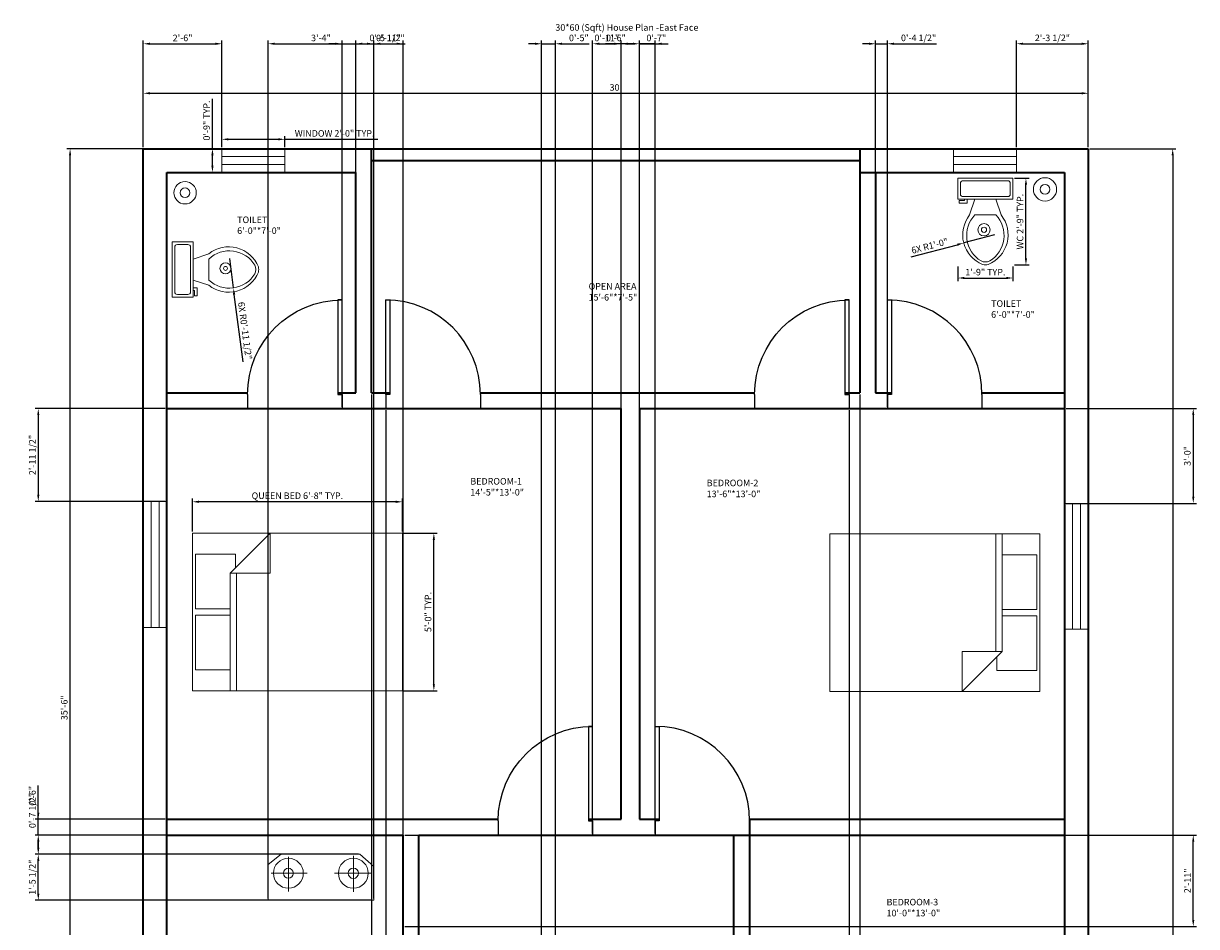
# Model space of a CAD drawing. Units: inches. Extents: x 2162 to 2610, y 1546 to 2356.
# Tile 3 of 3: x 2162 to 2609, y 2012 to 2356. Entities that reach past the tile are written whole.
import ezdxf

# ---------------------------------------------------------------- set-up
doc = ezdxf.new("R2010")
doc.units = ezdxf.units.IN
for name, color, linetype, lineweight in [('A-ANNO-DIMS', 2, 'Continuous', 18), ('A-ANNO-TEXT', 7, 'Continuous', 25), ('A-AREA-IDEN', 7, 'Continuous', 18), ('A-DOOR', 3, 'Continuous', 25), ('A-EQPM', 8, 'Continuous', 18), ('A-FLOR-FIXT', 9, 'Continuous', 18), ('A-FURN', 8, 'Continuous', 18), ('A-GLAZ', 4, 'Continuous', 18), ('A-WALL', 7, 'Continuous', 35)]:
    doc.layers.add(name, color=color, linetype=linetype, lineweight=lineweight)
doc.styles.get("Standard").update_dxf_attribs({"font": 'arial.ttf'})
doc.dimstyles.new('ISO-25', dxfattribs={"dimtxt": 2.5, "dimasz": 2.5, "dimexe": 1.25, "dimexo": 0.625, "dimtad": 1, "dimdec": 1, "dimlunit": 3, "dimtxsty": 'Standard', "dimcen": 2.5, "dimadec": 0, "dimazin": 0, "dimtfac": 1, "dimtdec": 1, "dimtmove": 0, "dimatfit": 3, "dimfxl": 1, "dimarcsym": 0})

# ---------------------------------------------------------------- blocks, each defined once
blk = doc.blocks.new('*U2')
for p, q in [((0, 0), (0, -6)), ((40, 0), (40, -6))]:
    blk.add_line(p, q)
blk.add_lwpolyline([(0, 0), (0, 40), (1.75, 40), (1.75, 0)], close=True)
blk.add_arc((0, 0), 40, 0, 90)
blk = doc.blocks.new('*D3')
at = {"layer": 'A-ANNO-DIMS', "color": 0, "lineweight": -2, "transparency": 16777216}
for p, q in [((2207.87, 2308.68), (2207.87, 2330.44)), ((2210.37, 2329.19), (2565.37, 2329.19)), ((2567.87, 2308.68), (2567.87, 2330.44))]:
    blk.add_line(p, q, dxfattribs=at)
at = {"layer": 'A-ANNO-DIMS', "color": 0, "transparency": 16777216}
for points in [[(2210.37, 2329.61), (2210.37, 2328.77), (2207.87, 2329.19)], [(2565.37, 2329.61), (2565.37, 2328.77), (2567.87, 2329.19)]]:
    blk.add_solid(points, dxfattribs=at)
at = {"layer": 'Defpoints', "color": 0, "transparency": 16777216}
for p in [(2567.87, 2329.19), (2207.87, 2308.05), (2567.87, 2308.05)]:
    blk.add_point(p, dxfattribs=at)
at = {"layer": 'A-ANNO-DIMS', "color": 0, "transparency": 16777216, "insert": (2387.87, 2331.09), "char_height": 2.5, "attachment_point": 5}
blk.add_mtext("30'", dxfattribs=at)
blk = doc.blocks.new('*D4')
at = {"layer": 'A-ANNO-DIMS', "color": 0, "lineweight": -2, "transparency": 16777216}
for p, q in [((2216.24, 2308.05), (2178.74, 2308.05)), ((2179.99, 1884.55), (2179.99, 2305.55)), ((2216.24, 1882.05), (2178.74, 1882.05))]:
    blk.add_line(p, q, dxfattribs=at)
at = {"layer": 'A-ANNO-DIMS', "color": 0, "transparency": 16777216}
for points in [[(2179.57, 2305.55), (2180.4, 2305.55), (2179.99, 2308.05)], [(2179.57, 1884.55), (2180.4, 1884.55), (2179.99, 1882.05)]]:
    blk.add_solid(points, dxfattribs=at)
at = {"layer": 'Defpoints', "color": 0, "transparency": 16777216}
for p in [(2179.99, 2308.05), (2216.87, 2308.05), (2216.87, 1882.05)]:
    blk.add_point(p, dxfattribs=at)
at = {"layer": 'A-ANNO-DIMS', "color": 0, "transparency": 16777216, "insert": (2178.09, 2095.05), "char_height": 2.5, "attachment_point": 5, "rotation": 90}
blk.add_mtext('35\'-6"', dxfattribs=at)
blk = doc.blocks.new('*D5')
at = {"layer": 'A-ANNO-DIMS', "color": 0, "lineweight": -2, "transparency": 16777216}
for p, q in [((2568.49, 2308.05), (2601.29, 2308.05)), ((2600.04, 2305.55), (2600.04, 1590.55)), ((2568.49, 1588.05), (2601.29, 1588.05))]:
    blk.add_line(p, q, dxfattribs=at)
at = {"layer": 'A-ANNO-DIMS', "color": 0, "transparency": 16777216}
for points in [[(2599.62, 2305.55), (2600.45, 2305.55), (2600.04, 2308.05)], [(2599.62, 1590.55), (2600.45, 1590.55), (2600.04, 1588.05)]]:
    blk.add_solid(points, dxfattribs=at)
at = {"layer": 'Defpoints', "color": 0, "transparency": 16777216}
for p in [(2567.87, 2308.05), (2567.87, 1588.05), (2600.04, 1588.05)]:
    blk.add_point(p, dxfattribs=at)
at = {"layer": 'A-ANNO-DIMS', "color": 0, "transparency": 16777216, "insert": (2598.14, 1948.05), "char_height": 2.5, "attachment_point": 5, "rotation": 90}
blk.add_mtext("60'", dxfattribs=at)
blk = doc.blocks.new('Bed - Queen')
for p, q in [((0, -80.00003), (0, 0)), ((0, 0), (59.99999, 0)), ((59.99999, 0), (59.99999, -80.00003)), ((7.99999, -1.2), (28.79998, -1.2)), ((7.99999, -14.4), (7.99999, -1.2)), ((28.79998, -1.2), (28.79998, -14.4)), ((31.19999, -1.2), (51.99999, -1.2)), ((31.19999, -14.4), (31.19999, -1.2)), ((51.99999, -1.2), (51.99999, -16.4)), ((0, -14.4), (44.8, -14.4)), ((44.8, -16.8), (0, -16.8)), ((59.99999, -29.6), (44.8, -14.4)), ((44.8, -14.4), (44.8, -29.6)), ((51.99999, -16.4), (46.79936, -16.4)), ((44.8, -29.6), (59.99999, -29.6)), ((59.99999, -80.00003), (0, -80.00003))]:
    blk.add_line(p, q)
blk = doc.blocks.new('Toilet - top')
for p, q in [((9.5, -6), (9.5, -2)), ((-10, -8.5), (-8, -8.5)), ((-10, -9.5), (-10, -8.5)), ((-8, -8.5), (-8, -8)), ((-7, -8), (-7, -9.5)), ((-4, -8), (-6, -14)), ((4, -8), (6, -14)), ((-7, -9.5), (-10, -9.5)), ((4, -14), (-4, -14))]:
    blk.add_line(p, q)
blk.add_lwpolyline([(10.5, -8), (10.5, 0), (-10.5, 0), (-10.5, -8)], close=True)
for points in [[(-9.5, -2), (-9.5, -6)], [(8.5, -1), (-8.5, -1)], [(-8.5, -7), (8.5, -7)]]:
    blk.add_lwpolyline(points)
for centre, radius, start, end in [((-8.62, -1.88), 0.884, 81.8699, 188.1301), ((8.62, -1.88), 0.884, 351.8699, 98.1301), ((-8.62, -6.12), 0.884, 171.8699, 278.1301), ((8.62, -6.12), 0.884, 261.8699, 8.1301), ((3.52, -21.58), 12.17, 141.4691, 247.9714), ((4.2, -21.82), 11.33, 136.3677, 238.9468), ((-3.52, -21.58), 12.17, 292.0284, 38.5307), ((-4.2, -21.82), 11.33, 301.053, 43.6321), ((0, -27.88), 4, 245.7318, 294.2682), ((0, -29), 4, 254.8605, 285.1395)]:
    blk.add_arc(centre, radius, start, end)
blk = doc.blocks.new('WIN-48IN')
for p, q in [((0, 0), (0, 48)), ((0, 48), (9, 48)), ((3, 0), (3, 48)), ((6, 48), (6, 0)), ((9, 48), (9, 0)), ((9, 0), (0, 0))]:
    blk.add_line(p, q)
blk = doc.blocks.new('WIN-24IN')
for p, q in [((0, 9), (24, 9)), ((0, 0), (0, 9)), ((24, 9), (24, 0)), ((0, 6), (24, 6)), ((24, 3), (0, 3)), ((24, 0), (0, 0))]:
    blk.add_line(p, q)
blk = doc.blocks.new('*D16')
at = {"layer": 'A-ANNO-DIMS', "color": 0, "lineweight": -2, "transparency": 16777216}
for p, q in [((2237.81, 2308.68), (2237.81, 2312.9)), ((2240.31, 2311.65), (2259.31, 2311.65)), ((2261.81, 2308.68), (2261.81, 2312.9)), ((2261.81, 2311.65), (2297.2, 2311.65))]:
    blk.add_line(p, q, dxfattribs=at)
at = {"layer": 'A-ANNO-DIMS', "color": 0, "transparency": 16777216}
for points in [[(2240.31, 2312.07), (2240.31, 2311.23), (2237.81, 2311.65)], [(2259.31, 2312.07), (2259.31, 2311.23), (2261.81, 2311.65)]]:
    blk.add_solid(points, dxfattribs=at)
at = {"layer": 'Defpoints', "color": 0, "transparency": 16777216}
for p in [(2261.81, 2311.65), (2237.81, 2308.05), (2261.81, 2308.05)]:
    blk.add_point(p, dxfattribs=at)
at = {"layer": 'A-ANNO-DIMS', "color": 0, "transparency": 16777216, "insert": (2280.76, 2313.57), "char_height": 2.5, "attachment_point": 5}
blk.add_mtext('WINDOW 2\'-0" TYP.', dxfattribs=at)
blk = doc.blocks.new('*D17')
at = {"layer": 'A-ANNO-DIMS', "color": 0, "lineweight": -2, "transparency": 16777216}
for p, q in [((2234.21, 2308.05), (2234.21, 2327.04)), ((2237.19, 2308.05), (2232.96, 2308.05)), ((2234.21, 2301.55), (2234.21, 2305.55)), ((2237.19, 2299.05), (2232.96, 2299.05))]:
    blk.add_line(p, q, dxfattribs=at)
at = {"layer": 'A-ANNO-DIMS', "color": 0, "transparency": 16777216}
for points in [[(2233.8, 2305.55), (2234.63, 2305.55), (2234.21, 2308.05)], [(2233.8, 2301.55), (2234.63, 2301.55), (2234.21, 2299.05)]]:
    blk.add_solid(points, dxfattribs=at)
at = {"layer": 'Defpoints', "color": 0, "transparency": 16777216}
for p in [(2234.21, 2308.05), (2237.81, 2308.05), (2237.81, 2299.05)]:
    blk.add_point(p, dxfattribs=at)
at = {"layer": 'A-ANNO-DIMS', "color": 0, "transparency": 16777216, "insert": (2232.31, 2318.8), "char_height": 2.5, "attachment_point": 5, "rotation": 90}
blk.add_mtext('0\'-9" TYP.', dxfattribs=at)
blk = doc.blocks.new('*D18')
at = {"layer": 'A-ANNO-DIMS', "color": 0, "lineweight": -2, "transparency": 16777216}
for p, q in [((2226.57, 2162.15), (2226.57, 2174.78)), ((2304.07, 2173.53), (2229.07, 2173.53)), ((2306.57, 2162.15), (2306.57, 2174.78))]:
    blk.add_line(p, q, dxfattribs=at)
at = {"layer": 'A-ANNO-DIMS', "color": 0, "transparency": 16777216}
for points in [[(2229.07, 2173.95), (2229.07, 2173.11), (2226.57, 2173.53)], [(2304.07, 2173.95), (2304.07, 2173.11), (2306.57, 2173.53)]]:
    blk.add_solid(points, dxfattribs=at)
at = {"layer": 'Defpoints', "color": 0, "transparency": 16777216}
for p in [(2226.57, 2173.53), (2226.57, 2161.53), (2306.57, 2161.53)]:
    blk.add_point(p, dxfattribs=at)
at = {"layer": 'A-ANNO-DIMS', "color": 0, "transparency": 16777216, "insert": (2266.57, 2175.52), "char_height": 2.5, "attachment_point": 5}
blk.add_mtext('QUEEN BED 6\'-8" TYP.', dxfattribs=at)
blk = doc.blocks.new('*D19')
at = {"layer": 'A-ANNO-DIMS', "color": 0, "lineweight": -2, "transparency": 16777216}
for p, q in [((2307.19, 2161.53), (2319.82, 2161.53)), ((2318.57, 2104.03), (2318.57, 2159.03)), ((2307.19, 2101.53), (2319.82, 2101.53))]:
    blk.add_line(p, q, dxfattribs=at)
at = {"layer": 'A-ANNO-DIMS', "color": 0, "transparency": 16777216}
for points in [[(2318.15, 2159.03), (2318.98, 2159.03), (2318.57, 2161.53)], [(2318.15, 2104.03), (2318.98, 2104.03), (2318.57, 2101.53)]]:
    blk.add_solid(points, dxfattribs=at)
at = {"layer": 'Defpoints', "color": 0, "transparency": 16777216}
for p in [(2306.57, 2161.53), (2318.57, 2161.53), (2306.57, 2101.53)]:
    blk.add_point(p, dxfattribs=at)
at = {"layer": 'A-ANNO-DIMS', "color": 0, "transparency": 16777216, "insert": (2316.67, 2131.53), "char_height": 2.5, "attachment_point": 5, "rotation": 90}
blk.add_mtext('5\'-0" TYP.', dxfattribs=at)
blk = doc.blocks.new('*D20')
at = {"layer": 'A-ANNO-DIMS', "color": 0, "lineweight": -2, "transparency": 16777216}
for p, q in [((2539.8, 2296.81), (2545.38, 2296.81)), ((2544.13, 2266.26), (2544.13, 2294.31)), ((2539.8, 2263.76), (2545.38, 2263.76))]:
    blk.add_line(p, q, dxfattribs=at)
at = {"layer": 'A-ANNO-DIMS', "color": 0, "transparency": 16777216}
for points in [[(2543.72, 2294.31), (2544.55, 2294.31), (2544.13, 2296.81)], [(2543.72, 2266.26), (2544.55, 2266.26), (2544.13, 2263.76)]]:
    blk.add_solid(points, dxfattribs=at)
at = {"layer": 'Defpoints', "color": 0, "transparency": 16777216}
for p in [(2539.18, 2296.81), (2544.13, 2296.81), (2539.18, 2263.76)]:
    blk.add_point(p, dxfattribs=at)
at = {"layer": 'A-ANNO-DIMS', "color": 0, "transparency": 16777216, "insert": (2542.22, 2280.28), "char_height": 2.5, "attachment_point": 5, "rotation": 90}
blk.add_mtext('WC 2\'-9" TYP.', dxfattribs=at)
blk = doc.blocks.new('*D21')
at = {"layer": 'A-ANNO-DIMS', "color": 0, "lineweight": -2, "transparency": 16777216}
for p, q in [((2518.18, 2263.14), (2518.18, 2257.55)), ((2539.18, 2263.14), (2539.18, 2257.55)), ((2520.68, 2258.8), (2536.68, 2258.8))]:
    blk.add_line(p, q, dxfattribs=at)
at = {"layer": 'A-ANNO-DIMS', "color": 0, "transparency": 16777216}
for points in [[(2520.68, 2259.22), (2520.68, 2258.39), (2518.18, 2258.8)], [(2536.68, 2259.22), (2536.68, 2258.39), (2539.18, 2258.8)]]:
    blk.add_solid(points, dxfattribs=at)
at = {"layer": 'Defpoints', "color": 0, "transparency": 16777216}
for p in [(2518.18, 2263.76), (2539.18, 2263.76), (2539.18, 2258.8)]:
    blk.add_point(p, dxfattribs=at)
at = {"layer": 'A-ANNO-DIMS', "color": 0, "transparency": 16777216, "insert": (2528.68, 2260.71), "char_height": 2.5, "attachment_point": 5}
blk.add_mtext('1\'-9" TYP.', dxfattribs=at)
blk = doc.blocks.new('*D27')
at = {"layer": 'A-ANNO-DIMS', "color": 0, "lineweight": -2, "transparency": 16777216}
for p, q in [((2216.24, 2209.05), (2166.62, 2209.05)), ((2167.87, 2206.55), (2167.87, 2176.19)), ((2216.24, 2173.69), (2166.62, 2173.69))]:
    blk.add_line(p, q, dxfattribs=at)
at = {"layer": 'A-ANNO-DIMS', "color": 0, "transparency": 16777216}
for points in [[(2167.45, 2206.55), (2168.28, 2206.55), (2167.87, 2209.05)], [(2167.45, 2176.19), (2168.28, 2176.19), (2167.87, 2173.69)]]:
    blk.add_solid(points, dxfattribs=at)
at = {"layer": 'Defpoints', "color": 0, "transparency": 16777216}
for p in [(2216.87, 2209.05), (2167.87, 2173.69), (2216.87, 2173.69)]:
    blk.add_point(p, dxfattribs=at)
at = {"layer": 'A-ANNO-DIMS', "color": 0, "transparency": 16777216, "insert": (2165.95, 2191.37), "char_height": 2.5, "attachment_point": 5, "rotation": 90}
blk.add_mtext('2\'-11 1/2"', dxfattribs=at)
blk = doc.blocks.new('*D30')
at = {"layer": 'A-ANNO-DIMS', "color": 0, "lineweight": -2, "transparency": 16777216}
for p, q in [((2559.49, 2209.05), (2609.12, 2209.05)), ((2607.87, 2206.55), (2607.87, 2175.44)), ((2559.49, 2172.94), (2609.12, 2172.94))]:
    blk.add_line(p, q, dxfattribs=at)
at = {"layer": 'A-ANNO-DIMS', "color": 0, "transparency": 16777216}
for points in [[(2607.45, 2206.55), (2608.28, 2206.55), (2607.87, 2209.05)], [(2607.45, 2175.44), (2608.28, 2175.44), (2607.87, 2172.94)]]:
    blk.add_solid(points, dxfattribs=at)
at = {"layer": 'Defpoints', "color": 0, "transparency": 16777216}
for p in [(2558.87, 2209.05), (2558.87, 2172.94), (2607.87, 2172.94)]:
    blk.add_point(p, dxfattribs=at)
at = {"layer": 'A-ANNO-DIMS', "color": 0, "transparency": 16777216, "insert": (2605.96, 2191), "char_height": 2.5, "attachment_point": 5, "rotation": 90}
blk.add_mtext('3\'-0"', dxfattribs=at)
blk = doc.blocks.new('*D35')
at = {"layer": 'A-ANNO-DIMS', "color": 0, "lineweight": -2, "transparency": 16777216}
for p, q in [((2207.87, 2308.68), (2207.87, 2349.3)), ((2210.37, 2348.05), (2235.31, 2348.05)), ((2237.81, 2308.68), (2237.81, 2349.3))]:
    blk.add_line(p, q, dxfattribs=at)
at = {"layer": 'A-ANNO-DIMS', "color": 0, "transparency": 16777216}
for points in [[(2210.37, 2348.47), (2210.37, 2347.63), (2207.87, 2348.05)], [(2235.31, 2348.47), (2235.31, 2347.63), (2237.81, 2348.05)]]:
    blk.add_solid(points, dxfattribs=at)
at = {"layer": 'Defpoints', "color": 0, "transparency": 16777216}
for p in [(2237.81, 2348.05), (2207.87, 2308.05), (2237.81, 2308.05)]:
    blk.add_point(p, dxfattribs=at)
at = {"layer": 'A-ANNO-DIMS', "color": 0, "transparency": 16777216, "insert": (2222.84, 2349.95), "char_height": 2.5, "attachment_point": 5}
blk.add_mtext('2\'-6"', dxfattribs=at)
blk = doc.blocks.new('*D36')
at = {"layer": 'A-ANNO-DIMS', "color": 0, "lineweight": -2, "transparency": 16777216}
for p, q in [((2540.53, 2308.68), (2540.53, 2349.3)), ((2543.03, 2348.05), (2565.37, 2348.05)), ((2567.87, 2308.68), (2567.87, 2349.3))]:
    blk.add_line(p, q, dxfattribs=at)
at = {"layer": 'A-ANNO-DIMS', "color": 0, "transparency": 16777216}
for points in [[(2543.03, 2348.47), (2543.03, 2347.63), (2540.53, 2348.05)], [(2565.37, 2348.47), (2565.37, 2347.63), (2567.87, 2348.05)]]:
    blk.add_solid(points, dxfattribs=at)
at = {"layer": 'Defpoints', "color": 0, "transparency": 16777216}
for p in [(2567.87, 2348.05), (2540.53, 2308.05), (2567.87, 2308.05)]:
    blk.add_point(p, dxfattribs=at)
at = {"layer": 'A-ANNO-DIMS', "color": 0, "transparency": 16777216, "insert": (2554.2, 2349.97), "char_height": 2.5, "attachment_point": 5}
blk.add_mtext('2\'-3 1/2"', dxfattribs=at)
blk = doc.blocks.new('*D41')
at = {"layer": 'A-ANNO-DIMS', "color": 0, "lineweight": -2, "transparency": 16777216}
for p, q in [((2307.49, 2046.55), (2609.12, 2046.55)), ((2607.87, 2014.19), (2607.87, 2044.05)), ((2307.49, 2011.69), (2609.12, 2011.69))]:
    blk.add_line(p, q, dxfattribs=at)
at = {"layer": 'A-ANNO-DIMS', "color": 0, "transparency": 16777216}
for points in [[(2607.45, 2044.05), (2608.28, 2044.05), (2607.87, 2046.55)], [(2607.45, 2014.19), (2608.28, 2014.19), (2607.87, 2011.69)]]:
    blk.add_solid(points, dxfattribs=at)
at = {"layer": 'Defpoints', "color": 0, "transparency": 16777216}
for p in [(2306.87, 2046.55), (2607.87, 2046.55), (2306.87, 2011.69)]:
    blk.add_point(p, dxfattribs=at)
at = {"layer": 'A-ANNO-DIMS', "color": 0, "transparency": 16777216, "insert": (2605.99, 2029.12), "char_height": 2.5, "attachment_point": 5, "rotation": 90}
blk.add_mtext('2\'-11"', dxfattribs=at)
blk = doc.blocks.new('*D42')
at = {"layer": 'A-ANNO-DIMS', "color": 0, "lineweight": -2, "transparency": 16777216}
for p, q in [((2255.46, 2022.36), (2255.46, 2349.3)), ((2257.96, 2348.05), (2293.14, 2348.05)), ((2295.64, 2022.36), (2295.64, 2349.3))]:
    blk.add_line(p, q, dxfattribs=at)
at = {"layer": 'A-ANNO-DIMS', "color": 0, "transparency": 16777216}
for points in [[(2257.96, 2348.47), (2257.96, 2347.63), (2255.46, 2348.05)], [(2293.14, 2348.47), (2293.14, 2347.63), (2295.64, 2348.05)]]:
    blk.add_solid(points, dxfattribs=at)
at = {"layer": 'Defpoints', "color": 0, "transparency": 16777216}
for p in [(2295.64, 2348.05), (2255.46, 2021.73), (2295.64, 2021.73)]:
    blk.add_point(p, dxfattribs=at)
at = {"layer": 'A-ANNO-DIMS', "color": 0, "transparency": 16777216, "insert": (2275.55, 2349.95), "char_height": 2.5, "attachment_point": 5}
blk.add_mtext('3\'-4"', dxfattribs=at)
blk = doc.blocks.new('*D43')
at = {"layer": 'A-ANNO-DIMS', "color": 0, "lineweight": -2, "transparency": 16777216}
for p, q in [((2289.8, 2039.22), (2166.62, 2039.22)), ((2167.87, 2024.23), (2167.87, 2036.72)), ((2295.02, 2021.73), (2166.62, 2021.73))]:
    blk.add_line(p, q, dxfattribs=at)
at = {"layer": 'A-ANNO-DIMS', "color": 0, "transparency": 16777216}
for points in [[(2167.45, 2036.72), (2168.28, 2036.72), (2167.87, 2039.22)], [(2167.45, 2024.23), (2168.28, 2024.23), (2167.87, 2021.73)]]:
    blk.add_solid(points, dxfattribs=at)
at = {"layer": 'Defpoints', "color": 0, "transparency": 16777216}
for p in [(2167.87, 2039.22), (2290.42, 2039.22), (2295.64, 2021.73)]:
    blk.add_point(p, dxfattribs=at)
at = {"layer": 'A-ANNO-DIMS', "color": 0, "transparency": 16777216, "insert": (2165.95, 2030.48), "char_height": 2.5, "attachment_point": 5, "rotation": 90}
blk.add_mtext('1\'-5 1/2"', dxfattribs=at)
blk = doc.blocks.new('*D45')
at = {"layer": 'A-ANNO-DIMS', "color": 0, "lineweight": -2, "transparency": 16777216}
for p, q in [((2295.64, 2022.36), (2295.64, 2349.3)), ((2298.14, 2348.05), (2304.37, 2348.05)), ((2306.87, 2012.32), (2306.87, 2349.3))]:
    blk.add_line(p, q, dxfattribs=at)
at = {"layer": 'A-ANNO-DIMS', "color": 0, "transparency": 16777216}
for points in [[(2298.14, 2348.47), (2298.14, 2347.63), (2295.64, 2348.05)], [(2304.37, 2348.47), (2304.37, 2347.63), (2306.87, 2348.05)]]:
    blk.add_solid(points, dxfattribs=at)
at = {"layer": 'Defpoints', "color": 0, "transparency": 16777216}
for p in [(2306.87, 2348.05), (2295.64, 2021.73), (2306.87, 2011.69)]:
    blk.add_point(p, dxfattribs=at)
at = {"layer": 'A-ANNO-DIMS', "color": 0, "transparency": 16777216, "insert": (2301.25, 2349.95), "char_height": 2.5, "attachment_point": 5}
blk.add_mtext('0\'-11"', dxfattribs=at)
blk = doc.blocks.new('*D46')
at = {"layer": 'A-ANNO-DIMS', "color": 0, "lineweight": -2, "transparency": 16777216}
for p, q in [((2167.87, 2046.55), (2167.87, 2062.77)), ((2306.24, 2046.55), (2166.62, 2046.55)), ((2167.87, 2041.72), (2167.87, 2044.05)), ((2289.8, 2039.22), (2166.62, 2039.22))]:
    blk.add_line(p, q, dxfattribs=at)
at = {"layer": 'A-ANNO-DIMS', "color": 0, "transparency": 16777216}
for points in [[(2167.45, 2044.05), (2168.28, 2044.05), (2167.87, 2046.55)], [(2167.45, 2041.72), (2168.28, 2041.72), (2167.87, 2039.22)]]:
    blk.add_solid(points, dxfattribs=at)
at = {"layer": 'Defpoints', "color": 0, "transparency": 16777216}
for p in [(2167.87, 2046.55), (2306.87, 2046.55), (2290.42, 2039.22)]:
    blk.add_point(p, dxfattribs=at)
at = {"layer": 'A-ANNO-DIMS', "color": 0, "transparency": 16777216, "insert": (2165.95, 2055.91), "char_height": 2.5, "attachment_point": 5, "rotation": 90}
blk.add_mtext('0\'-7 1/2"', dxfattribs=at)
blk = doc.blocks.new('*D50')
at = {"layer": 'A-ANNO-DIMS', "color": 0, "lineweight": -2, "transparency": 16777216}
for p, q in [((2357.13, 2348.05), (2354.63, 2348.05)), ((2359.63, 1882.68), (2359.63, 2349.3)), ((2359.63, 2348.05), (2364.87, 2348.05)), ((2364.87, 1882.68), (2364.87, 2349.3)), ((2367.37, 2348.05), (2377.76, 2348.05))]:
    blk.add_line(p, q, dxfattribs=at)
at = {"layer": 'A-ANNO-DIMS', "color": 0, "transparency": 16777216}
for points in [[(2357.13, 2348.47), (2357.13, 2347.63), (2359.63, 2348.05)], [(2367.37, 2348.47), (2367.37, 2347.63), (2364.87, 2348.05)]]:
    blk.add_solid(points, dxfattribs=at)
at = {"layer": 'Defpoints', "color": 0, "transparency": 16777216}
for p in [(2364.87, 2348.05), (2359.63, 1882.05), (2364.87, 1882.05)]:
    blk.add_point(p, dxfattribs=at)
at = {"layer": 'A-ANNO-DIMS', "color": 0, "transparency": 16777216, "insert": (2373.81, 2349.95), "char_height": 2.5, "attachment_point": 5}
blk.add_mtext('0\'-5"', dxfattribs=at)
blk = doc.blocks.new('*D51')
at = {"layer": 'A-ANNO-DIMS', "color": 0, "lineweight": -2, "transparency": 16777216}
for p, q in [((2389.87, 2053.18), (2389.87, 2349.3)), ((2392.37, 2348.05), (2394.37, 2348.05)), ((2396.87, 2053.18), (2396.87, 2349.3)), ((2396.87, 2348.05), (2407.26, 2348.05))]:
    blk.add_line(p, q, dxfattribs=at)
at = {"layer": 'A-ANNO-DIMS', "color": 0, "transparency": 16777216}
for points in [[(2392.37, 2348.47), (2392.37, 2347.63), (2389.87, 2348.05)], [(2394.37, 2348.47), (2394.37, 2347.63), (2396.87, 2348.05)]]:
    blk.add_solid(points, dxfattribs=at)
at = {"layer": 'Defpoints', "color": 0, "transparency": 16777216}
for p in [(2396.87, 2348.05), (2389.87, 2052.55), (2396.87, 2052.55)]:
    blk.add_point(p, dxfattribs=at)
at = {"layer": 'A-ANNO-DIMS', "color": 0, "transparency": 16777216, "insert": (2403.31, 2349.95), "char_height": 2.5, "attachment_point": 5}
blk.add_mtext('0\'-7"', dxfattribs=at)
blk = doc.blocks.new('*D52')
at = {"layer": 'A-ANNO-DIMS', "color": 0, "lineweight": -2, "transparency": 16777216}
for p, q in [((2167.87, 2055.05), (2167.87, 2065.45)), ((2216.24, 2052.55), (2166.62, 2052.55)), ((2167.87, 2046.55), (2167.87, 2052.55)), ((2216.24, 2046.55), (2166.62, 2046.55)), ((2167.87, 2044.05), (2167.87, 2041.55))]:
    blk.add_line(p, q, dxfattribs=at)
at = {"layer": 'A-ANNO-DIMS', "color": 0, "transparency": 16777216}
for points in [[(2167.45, 2055.05), (2168.28, 2055.05), (2167.87, 2052.55)], [(2167.45, 2044.05), (2168.28, 2044.05), (2167.87, 2046.55)]]:
    blk.add_solid(points, dxfattribs=at)
at = {"layer": 'Defpoints', "color": 0, "transparency": 16777216}
for p in [(2167.87, 2052.55), (2216.87, 2052.55), (2216.87, 2046.55)]:
    blk.add_point(p, dxfattribs=at)
at = {"layer": 'A-ANNO-DIMS', "color": 0, "transparency": 16777216, "insert": (2165.97, 2061.5), "char_height": 2.5, "attachment_point": 5, "rotation": 90}
blk.add_mtext('0\'-6"', dxfattribs=at)
blk = doc.blocks.new('*D53')
at = {"layer": 'A-ANNO-DIMS', "color": 0, "lineweight": -2, "transparency": 16777216}
for p, q in [((2379.05, 2047.18), (2379.05, 2349.3)), ((2381.55, 2348.05), (2387.37, 2348.05)), ((2389.87, 2053.18), (2389.87, 2349.3))]:
    blk.add_line(p, q, dxfattribs=at)
at = {"layer": 'A-ANNO-DIMS', "color": 0, "transparency": 16777216}
for points in [[(2381.55, 2348.47), (2381.55, 2347.63), (2379.05, 2348.05)], [(2387.37, 2348.47), (2387.37, 2347.63), (2389.87, 2348.05)]]:
    blk.add_solid(points, dxfattribs=at)
at = {"layer": 'Defpoints', "color": 0, "transparency": 16777216}
for p in [(2389.87, 2348.05), (2389.87, 2052.55), (2379.05, 2046.55)]:
    blk.add_point(p, dxfattribs=at)
at = {"layer": 'A-ANNO-DIMS', "color": 0, "transparency": 16777216, "insert": (2384.46, 2349.95), "char_height": 2.5, "attachment_point": 5}
blk.add_mtext('0\'-11"', dxfattribs=at)
blk = doc.blocks.new('*D54')
at = {"layer": 'A-ANNO-DIMS', "color": 0, "lineweight": -2, "transparency": 16777216}
for p, q in [((2394.37, 2348.05), (2383.97, 2348.05)), ((2396.87, 2053.18), (2396.87, 2349.3)), ((2402.87, 2348.05), (2396.87, 2348.05)), ((2402.87, 2047.18), (2402.87, 2349.3)), ((2405.37, 2348.05), (2407.87, 2348.05))]:
    blk.add_line(p, q, dxfattribs=at)
at = {"layer": 'A-ANNO-DIMS', "color": 0, "transparency": 16777216}
for points in [[(2394.37, 2348.47), (2394.37, 2347.63), (2396.87, 2348.05)], [(2405.37, 2348.47), (2405.37, 2347.63), (2402.87, 2348.05)]]:
    blk.add_solid(points, dxfattribs=at)
at = {"layer": 'Defpoints', "color": 0, "transparency": 16777216}
for p in [(2396.87, 2348.05), (2396.87, 2052.55), (2402.87, 2046.55)]:
    blk.add_point(p, dxfattribs=at)
at = {"layer": 'A-ANNO-DIMS', "color": 0, "transparency": 16777216, "insert": (2387.92, 2349.95), "char_height": 2.5, "attachment_point": 5}
blk.add_mtext('0\'-6"', dxfattribs=at)
blk = doc.blocks.new('*D55')
at = {"layer": 'A-ANNO-DIMS', "color": 0, "lineweight": -2, "transparency": 16777216}
for p, q in [((2281.09, 2348.05), (2278.59, 2348.05)), ((2283.59, 2209.68), (2283.59, 2349.3)), ((2283.59, 2348.05), (2288.87, 2348.05)), ((2288.87, 2215.68), (2288.87, 2349.3)), ((2291.37, 2348.05), (2307.59, 2348.05))]:
    blk.add_line(p, q, dxfattribs=at)
at = {"layer": 'A-ANNO-DIMS', "color": 0, "transparency": 16777216}
for points in [[(2281.09, 2348.47), (2281.09, 2347.63), (2283.59, 2348.05)], [(2291.37, 2348.47), (2291.37, 2347.63), (2288.87, 2348.05)]]:
    blk.add_solid(points, dxfattribs=at)
at = {"layer": 'Defpoints', "color": 0, "transparency": 16777216}
for p in [(2288.87, 2348.05), (2288.87, 2215.05), (2283.59, 2209.05)]:
    blk.add_point(p, dxfattribs=at)
at = {"layer": 'A-ANNO-DIMS', "color": 0, "transparency": 16777216, "insert": (2300.73, 2349.97), "char_height": 2.5, "attachment_point": 5}
blk.add_mtext('0\'-5 1/2"', dxfattribs=at)
blk = doc.blocks.new('*D56')
at = {"layer": 'A-ANNO-DIMS', "color": 0, "lineweight": -2, "transparency": 16777216}
for p, q in [((2294.87, 2214.43), (2294.87, 1546.8)), ((2300.28, 2208.43), (2300.28, 1546.8)), ((2292.37, 1548.05), (2289.87, 1548.05)), ((2294.87, 1548.05), (2300.28, 1548.05)), ((2302.78, 1548.05), (2319.01, 1548.05))]:
    blk.add_line(p, q, dxfattribs=at)
at = {"layer": 'A-ANNO-DIMS', "color": 0, "transparency": 16777216}
for points in [[(2292.37, 1548.47), (2292.37, 1547.63), (2294.87, 1548.05)], [(2302.78, 1548.47), (2302.78, 1547.63), (2300.28, 1548.05)]]:
    blk.add_solid(points, dxfattribs=at)
at = {"layer": 'Defpoints', "color": 0, "transparency": 16777216}
for p in [(2294.87, 2215.05), (2300.28, 2209.05), (2300.28, 1548.05)]:
    blk.add_point(p, dxfattribs=at)
at = {"layer": 'A-ANNO-DIMS', "color": 0, "transparency": 16777216, "insert": (2312.14, 1549.97), "char_height": 2.5, "attachment_point": 5}
blk.add_mtext('0\'-5 1/2"', dxfattribs=at)
blk = doc.blocks.new('*D57')
at = {"layer": 'A-ANNO-DIMS', "color": 0, "lineweight": -2, "transparency": 16777216}
for p, q in [((2480.87, 2214.43), (2480.87, 1546.8)), ((2476.76, 2208.43), (2476.76, 1546.8)), ((2474.26, 1548.05), (2471.76, 1548.05)), ((2476.76, 1548.05), (2480.87, 1548.05)), ((2483.37, 1548.05), (2493.76, 1548.05))]:
    blk.add_line(p, q, dxfattribs=at)
at = {"layer": 'A-ANNO-DIMS', "color": 0, "transparency": 16777216}
for points in [[(2474.26, 1548.47), (2474.26, 1547.63), (2476.76, 1548.05)], [(2483.37, 1548.47), (2483.37, 1547.63), (2480.87, 1548.05)]]:
    blk.add_solid(points, dxfattribs=at)
at = {"layer": 'Defpoints', "color": 0, "transparency": 16777216}
for p in [(2480.87, 2215.05), (2476.76, 2209.05), (2480.87, 1548.05)]:
    blk.add_point(p, dxfattribs=at)
at = {"layer": 'A-ANNO-DIMS', "color": 0, "transparency": 16777216, "insert": (2489.81, 1549.95), "char_height": 2.5, "attachment_point": 5}
blk.add_mtext('0\'-4"', dxfattribs=at)
blk = doc.blocks.new('*D58')
at = {"layer": 'A-ANNO-DIMS', "color": 0, "lineweight": -2, "transparency": 16777216}
for p, q in [((2484.37, 2348.05), (2481.87, 2348.05)), ((2486.87, 2215.68), (2486.87, 2349.3)), ((2486.87, 2348.05), (2491.37, 2348.05)), ((2491.37, 2209.68), (2491.37, 2349.3)), ((2493.87, 2348.05), (2510.09, 2348.05))]:
    blk.add_line(p, q, dxfattribs=at)
at = {"layer": 'A-ANNO-DIMS', "color": 0, "transparency": 16777216}
for points in [[(2484.37, 2348.47), (2484.37, 2347.63), (2486.87, 2348.05)], [(2493.87, 2348.47), (2493.87, 2347.63), (2491.37, 2348.05)]]:
    blk.add_solid(points, dxfattribs=at)
at = {"layer": 'Defpoints', "color": 0, "transparency": 16777216}
for p in [(2491.37, 2348.05), (2486.87, 2215.05), (2491.37, 2209.05)]:
    blk.add_point(p, dxfattribs=at)
at = {"layer": 'A-ANNO-DIMS', "color": 0, "transparency": 16777216, "insert": (2503.23, 2349.97), "char_height": 2.5, "attachment_point": 5}
blk.add_mtext('0\'-4 1/2"', dxfattribs=at)
blk = doc.blocks.new('*D62')
at = {"layer": 'A-ANNO-DIMS', "color": 0, "lineweight": -2, "transparency": 16777216}
for p, q in [((2532.2, 2275.23), (2520.43, 2272.14)), ((2500.43, 2266.88), (2518.01, 2271.5))]:
    blk.add_line(p, q, dxfattribs=at)
at = {"layer": 'A-ANNO-DIMS', "color": 0, "transparency": 16777216}
blk.add_solid([(2517.9, 2271.9), (2518.12, 2271.1), (2520.43, 2272.14)], dxfattribs=at)
at = {"layer": 'Defpoints', "color": 0, "transparency": 16777216}
for p in [(2532.2, 2275.23), (2520.43, 2272.14)]:
    blk.add_point(p, dxfattribs=at)
at = {"layer": 'A-ANNO-DIMS', "color": 0, "transparency": 16777216, "insert": (2507.53, 2270.71), "char_height": 2.5, "attachment_point": 5, "rotation": 14.72}
blk.add_mtext('6X R1\'-0"', dxfattribs=at)
blk = doc.blocks.new('*D63')
at = {"layer": 'A-ANNO-DIMS', "color": 0, "lineweight": -2, "transparency": 16777216}
for p, q in [((2240.66, 2266.24), (2242.17, 2255.01)), ((2245.96, 2226.82), (2242.51, 2252.53))]:
    blk.add_line(p, q, dxfattribs=at)
at = {"layer": 'A-ANNO-DIMS', "color": 0, "transparency": 16777216}
blk.add_solid([(2242.92, 2252.59), (2242.09, 2252.47), (2242.17, 2255.01)], dxfattribs=at)
at = {"layer": 'Defpoints', "color": 0, "transparency": 16777216}
for p in [(2240.66, 2266.24), (2242.17, 2255.01)]:
    blk.add_point(p, dxfattribs=at)
at = {"layer": 'A-ANNO-DIMS', "color": 0, "transparency": 16777216, "insert": (2246.3, 2238.69), "char_height": 2.5, "attachment_point": 5, "rotation": 277.6561}
blk.add_mtext('6X R0\'-11 1/2"', dxfattribs=at)

msp = doc.modelspace()

# ---------------------------------------------------------------- linework, layer by layer
at = {"layer": 'A-EQPM'}
for p, q in [((2255.46, 2035.34), (2260.45, 2039.22)), ((2263.14, 2032), (2263.14, 2038.26)), ((2287.89, 2032), (2287.89, 2038.64)), ((2290.42, 2039.22), (2295.64, 2034.52)), ((2263.14, 2032), (2256.58, 2032)), ((2263.14, 2032), (2263.14, 2025.05)), ((2263.14, 2032), (2270.27, 2032)), ((2287.89, 2032), (2280.75, 2032)), ((2287.89, 2032), (2294.62, 2032)), ((2287.89, 2032), (2287.89, 2024.94))]:
    msp.add_line(p, q, dxfattribs=at)
for points in [[(2260.45, 2039.22), (2290.42, 2039.22)], [(2295.64, 2034.52), (2295.64, 2021.73), (2255.46, 2021.73), (2255.46, 2035.34)]]:
    msp.add_lwpolyline(points, dxfattribs=at)
for centre, radius in [((2263.14, 2032), 5.69), ((2263.14, 2032), 1.9), ((2287.89, 2032), 5.69), ((2287.89, 2032), 1.97)]:
    msp.add_circle(centre, radius, dxfattribs=at)
at = {"layer": 'A-FLOR-FIXT'}
for centre, radius in [((2223.77, 2291.3), 4.28), ((2223.77, 2291.3), 1.81), ((2551.39, 2292.57), 4.43), ((2551.39, 2292.57), 1.82), ((2528.15, 2277.17), 2.34), ((2528.15, 2277.17), 0.995), ((2239.19, 2262.47), 2.12), ((2239.19, 2262.47), 0.752)]:
    msp.add_circle(centre, radius, dxfattribs=at)
at = {"layer": 'A-WALL'}
for p, q in [((2207.87, 2308.05), (2567.87, 2308.05)), ((2207.87, 1588.05), (2207.87, 2308.05)), ((2294.87, 2215.05), (2294.87, 2308.05)), ((2480.87, 2308.05), (2480.87, 2215.05)), ((2567.87, 2308.05), (2567.87, 1588.05)), ((2294.87, 2303.55), (2480.87, 2303.55)), ((2216.87, 2299.05), (2288.87, 2299.05)), ((2216.87, 1588.05), (2216.87, 2299.05)), ((2288.87, 2215.05), (2288.87, 2299.05)), ((2480.87, 2299.05), (2558.87, 2299.05)), ((2486.87, 2299.05), (2486.87, 2215.05)), ((2558.87, 2299.05), (2558.87, 1595.05)), ((2216.87, 2215.05), (2247.6, 2215.05)), ((2282.02, 2215.05), (2288.87, 2215.05)), ((2294.87, 2215.05), (2301.86, 2215.05)), ((2336.28, 2215.05), (2440.76, 2215.05)), ((2475.18, 2215.05), (2480.87, 2215.05)), ((2486.87, 2215.05), (2492.94, 2215.05)), ((2527.36, 2215.05), (2558.87, 2215.05)), ((2216.87, 2209.05), (2389.87, 2209.05)), ((2389.87, 2052.55), (2389.87, 2209.05)), ((2396.87, 2209.05), (2558.87, 2209.05)), ((2396.87, 2209.05), (2396.87, 2052.55)), ((2216.87, 2052.55), (2343.06, 2052.55)), ((2377.48, 2052.55), (2389.87, 2052.55)), ((2396.87, 2052.55), (2404.44, 2052.55)), ((2438.86, 2052.55), (2558.87, 2052.55)), ((2438.87, 2052.55), (2438.87, 1932.84)), ((2216.87, 2046.55), (2306.87, 2046.55)), ((2306.87, 1979.36), (2306.87, 2046.55)), ((2312.87, 2046.55), (2558.87, 2046.55)), ((2312.87, 1979.36), (2312.87, 2046.55)), ((2432.87, 1882.05), (2432.87, 2046.55))]:
    msp.add_line(p, q, dxfattribs=at)

# ---------------------------------------------------------------- block references
at = {"layer": 'A-DOOR', "yscale": 0.9, "zscale": 0.9}
for p, xscale in [((2283.59, 2214.45), -0.9), ((2300.28, 2214.45), 0.9), ((2476.76, 2214.45), -0.9), ((2491.37, 2214.45), 0.9), ((2379.05, 2051.95), -0.9), ((2402.87, 2051.95), 0.9)]:
    msp.add_blockref('*U2', p, dxfattribs=dict(at, xscale=xscale))
at = {"layer": 'A-FLOR-FIXT'}
msp.add_blockref('Toilet - top', (2528.68, 2296.81), dxfattribs=at)
at = {"layer": 'A-FLOR-FIXT', "rotation": 90}
msp.add_blockref('Toilet - top', (2218.85, 2262.04), dxfattribs=at)
at = {"layer": 'A-FURN'}
for p, rotation in [((2226.57, 2101.53), 90), ((2549.47, 2161.28), 270)]:
    msp.add_blockref('Bed - Queen', p, dxfattribs=dict(at, rotation=rotation))
at = {"layer": 'A-GLAZ'}
for name, p in [('WIN-24IN', (2237.81, 2299.05)), ('WIN-24IN', (2516.53, 2299.05)), ('WIN-48IN', (2207.87, 2125.69)), ('WIN-48IN', (2558.87, 2124.94))]:
    msp.add_blockref(name, p, dxfattribs=at)

# ---------------------------------------------------------------- texts
at = {"layer": 'A-ANNO-TEXT', "insert": (2364.85, 2355.5), "char_height": 2.5, "attachment_point": 1}
msp.add_mtext_dynamic_manual_height_columns('30*60 (Sqft) House Plan -East Face', width=361.1178, gutter_width=12.5, heights=[0], dxfattribs=at)
at = {"layer": 'A-AREA-IDEN', "char_height": 2.5, "attachment_point": 1}
for s, width, insert in [('TOILET\\P6\'-0"*7\'-0"', 32.5546, (2243.64, 2282.23)), ('OPEN AREA\\P15\'-6"*7\'-5"', 76.413, (2377.51, 2256.88)), ('TOILET\\P6\'-0"*7\'-0"', 39.4303, (2530.87, 2250.31)), ('BEDROOM-1\\P14\'-5"*13\'-0"', 73.709, (2332.46, 2182.59)), ('BEDROOM-2\\P13\'-6"*13\'-0"', 41.4283, (2422.52, 2181.96)), ('BEDROOM-3\\P10\'-0"*13\'-0"', 63.0728, (2491.02, 2022.25))]:
    msp.add_mtext_dynamic_manual_height_columns(s, width=width, gutter_width=12.5, heights=[0], dxfattribs=dict(at, insert=insert))

# ---------------------------------------------------------------- dimensions: what is measured, and where the dimension line sits
at = {"layer": 'A-ANNO-DIMS'}
for base, p1, p2, override, picture, middle in [((2237.81, 2348.05), (2207.87, 2308.05), (2237.81, 2308.05), {"dimdec": 1, "dimlfac": 1, "dimrnd": 0, "dimzin": 1, "dimdsep": 46, "dimlunit": 4, "dimfrac": 2}, '*D35', (2222.84, 2349.95)), ((2295.64, 2348.05), (2255.46, 2021.73), (2295.64, 2021.73), {"dimdec": 1, "dimlfac": 1, "dimrnd": 0, "dimzin": 1, "dimdsep": 46, "dimlunit": 4, "dimfrac": 2}, '*D42', (2275.55, 2349.95)), ((2288.87, 2348.05), (2283.59, 2209.05), (2288.87, 2215.05), {"dimdec": 1, "dimlfac": 1, "dimrnd": 0, "dimzin": 1, "dimdsep": 46, "dimlunit": 4, "dimfrac": 2}, '*D55', (2300.73, 2349.97)), ((2306.87, 2348.05), (2295.64, 2021.73), (2306.87, 2011.69), {"dimdec": 1, "dimlfac": 1, "dimrnd": 0, "dimzin": 1, "dimdsep": 46, "dimlunit": 4, "dimfrac": 2}, '*D45', (2301.25, 2349.95)), ((2364.87, 2348.05), (2359.63, 1882.05), (2364.87, 1882.05), {"dimdec": 1, "dimlfac": 1, "dimrnd": 0, "dimzin": 1, "dimdsep": 46, "dimlunit": 4, "dimfrac": 2}, '*D50', (2373.81, 2349.95)), ((2389.87, 2348.05), (2379.05, 2046.55), (2389.87, 2052.55), {"dimdec": 1, "dimlfac": 1, "dimrnd": 0, "dimzin": 1, "dimdsep": 46, "dimlunit": 4, "dimfrac": 2}, '*D53', (2384.46, 2349.95)), ((2396.87, 2348.05), (2402.87, 2046.55), (2396.87, 2052.55), {"dimdec": 1, "dimlfac": 1, "dimrnd": 0, "dimzin": 1, "dimdsep": 46, "dimlunit": 4, "dimfrac": 2}, '*D54', (2387.92, 2349.95)), ((2396.87, 2348.05), (2389.87, 2052.55), (2396.87, 2052.55), {"dimdec": 1, "dimlfac": 1, "dimrnd": 0, "dimzin": 1, "dimdsep": 46, "dimlunit": 4, "dimfrac": 2}, '*D51', (2403.31, 2349.95)), ((2491.37, 2348.05), (2486.87, 2215.05), (2491.37, 2209.05), {"dimdec": 1, "dimlfac": 1, "dimrnd": 0, "dimzin": 1, "dimdsep": 46, "dimlunit": 4, "dimfrac": 2}, '*D58', (2503.23, 2349.97)), ((2567.87, 2348.05), (2540.53, 2308.05), (2567.87, 2308.05), {"dimdec": 1, "dimlfac": 1, "dimrnd": 0, "dimzin": 1, "dimdsep": 46, "dimlunit": 4, "dimfrac": 2}, '*D36', (2554.2, 2349.97)), ((2567.87, 2329.19), (2207.87, 2308.05), (2567.87, 2308.05), {"dimclrd": 0, "dimclre": 0, "dimclrt": 0}, '*D3', (2387.87, 2331.09)), ((2300.28, 1548.05), (2294.87, 2215.05), (2300.28, 2209.05), {"dimdec": 1, "dimlfac": 1, "dimrnd": 0, "dimzin": 1, "dimdsep": 46, "dimlunit": 4, "dimfrac": 2}, '*D56', (2312.14, 1549.97)), ((2480.87, 1548.05), (2476.76, 2209.05), (2480.87, 2215.05), {"dimdec": 1, "dimlfac": 1, "dimrnd": 0, "dimzin": 1, "dimdsep": 46, "dimlunit": 4, "dimfrac": 2}, '*D57', (2489.81, 1549.95))]:
    dim = msp.add_linear_dim(base=base, p1=p1, p2=p2, dimstyle='ISO-25', override=override, dxfattribs=at)
    dim.commit()
    dim.dimension.update_dxf_attribs({"geometry": picture, "text_midpoint": middle})
for base, p1, p2, angle, text, picture, middle in [((2234.21, 2308.05), (2237.81, 2299.05), (2237.81, 2308.05), 90, '<> TYP.', '*D17', (2232.31, 2318.8)), ((2544.1343, 2296.8077), (2539.1774, 2263.7614), (2539.1774, 2296.8077), 90, 'WC <> TYP.', '*D20', (2542.2167, 2280.2846)), ((2226.57, 2173.53), (2306.57, 2161.53), (2226.57, 2161.53), 180, 'QUEEN BED <> TYP.', '*D18', (2266.57, 2175.52)), ((2318.57, 2161.53), (2306.57, 2101.53), (2306.57, 2161.53), 90, '<> TYP.', '*D19', (2316.67, 2131.53))]:
    dim = msp.add_linear_dim(base=base, p1=p1, p2=p2, angle=angle, text=text, dimstyle='ISO-25', override={"dimdec": 1, "dimlfac": 1, "dimrnd": 0, "dimzin": 1, "dimdsep": 46, "dimlunit": 4, "dimfrac": 2}, dxfattribs=at)
    dim.commit()
    dim.dimension.update_dxf_attribs({"geometry": picture, "text_midpoint": middle})
for base, p1, p2, text, picture, middle in [((2261.81, 2311.65), (2237.81, 2308.05), (2261.81, 2308.05), 'WINDOW <> TYP.', '*D16', (2280.76, 2313.57)), ((2539.18, 2258.8), (2518.18, 2263.76), (2539.18, 2263.76), '<> TYP.', '*D21', (2528.68, 2260.71))]:
    dim = msp.add_linear_dim(base=base, p1=p1, p2=p2, text=text, dimstyle='ISO-25', override={"dimdec": 1, "dimlfac": 1, "dimrnd": 0, "dimzin": 1, "dimdsep": 46, "dimlunit": 4, "dimfrac": 2}, dxfattribs=at)
    dim.commit()
    dim.dimension.update_dxf_attribs({"geometry": picture, "text_midpoint": middle})
for base, p1, p2, override, picture, middle in [((2179.99, 2308.05), (2216.87, 1882.05), (2216.87, 2308.05), {"dimclrd": 0, "dimclre": 0, "dimclrt": 0}, '*D4', (2178.09, 2095.05)), ((2600.04, 1588.05), (2567.87, 2308.05), (2567.87, 1588.05), {"dimclrd": 0, "dimclre": 0, "dimclrt": 0}, '*D5', (2598.14, 1948.05)), ((2167.87, 2173.69), (2216.87, 2209.05), (2216.87, 2173.69), {"dimdec": 1, "dimlfac": 1, "dimrnd": 0, "dimzin": 1, "dimdsep": 46, "dimlunit": 4, "dimfrac": 2}, '*D27', (2165.95, 2191.37)), ((2607.87, 2172.94), (2558.87, 2209.05), (2558.87, 2172.94), {"dimdec": 1, "dimlfac": 1, "dimrnd": 0, "dimzin": 1, "dimdsep": 46, "dimlunit": 4, "dimfrac": 2}, '*D30', (2605.96, 2191)), ((2167.87, 2052.55), (2216.87, 2046.55), (2216.87, 2052.55), {"dimdec": 1, "dimlfac": 1, "dimrnd": 0, "dimzin": 1, "dimdsep": 46, "dimlunit": 4, "dimfrac": 2}, '*D52', (2165.97, 2061.5)), ((2167.87, 2046.55), (2290.42, 2039.22), (2306.87, 2046.55), {"dimdec": 1, "dimlfac": 1, "dimrnd": 0, "dimzin": 1, "dimdsep": 46, "dimlunit": 4, "dimfrac": 2}, '*D46', (2165.95, 2055.91)), ((2607.87, 2046.55), (2306.87, 2011.69), (2306.87, 2046.55), {"dimdec": 1, "dimlfac": 1, "dimrnd": 0, "dimzin": 1, "dimdsep": 46, "dimlunit": 4, "dimfrac": 2}, '*D41', (2605.99, 2029.12)), ((2167.87, 2039.22), (2295.64, 2021.73), (2290.42, 2039.22), {"dimdec": 1, "dimlfac": 1, "dimrnd": 0, "dimzin": 1, "dimdsep": 46, "dimlunit": 4, "dimfrac": 2}, '*D43', (2165.95, 2030.48))]:
    dim = msp.add_linear_dim(base=base, p1=p1, p2=p2, angle=90, dimstyle='ISO-25', override=override, dxfattribs=at)
    dim.commit()
    dim.dimension.update_dxf_attribs({"geometry": picture, "text_midpoint": middle})
for center, mpoint, picture, middle in [((2532.2, 2275.23), (2520.43, 2272.14), '*D62', (2507.53, 2270.71)), ((2240.66, 2266.24), (2242.17, 2255.01), '*D63', (2246.3, 2238.69))]:
    dim = msp.add_radius_dim(center=center, mpoint=mpoint, text='6X <>', dimstyle='ISO-25', override={"dimdec": 1, "dimlfac": 1, "dimrnd": 0, "dimzin": 1, "dimdsep": 46, "dimlunit": 4, "dimfrac": 2}, dxfattribs=at)
    dim.commit()
    dim.dimension.update_dxf_attribs({"geometry": picture, "text_midpoint": middle})

doc.saveas('drawing.dxf')
